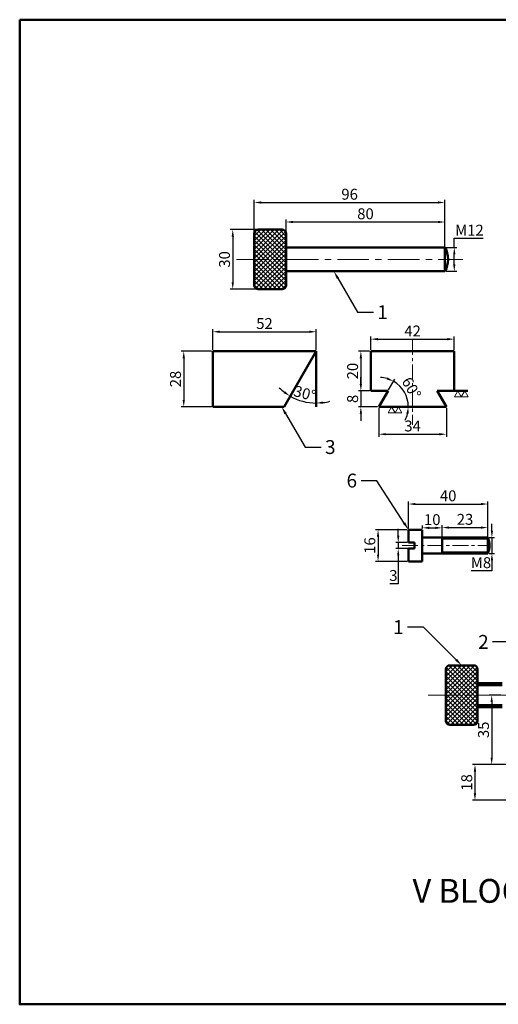
# Model space of a CAD drawing. Units: millimetres. Extents: x 10 to 613, y -226 to 271.
# Tile 1 of 4: x 10 to 251, y -226 to 271. Entities that reach past the tile are written whole.
import ezdxf
from ezdxf import colors
from ezdxf.entities.mleader import LeaderData, LeaderLine
from ezdxf.math import Vec2, Vec3

# ---------------------------------------------------------------- set-up
doc = ezdxf.new("R2010")
doc.units = ezdxf.units.MM
doc.header["$LTSCALE"] = 0.5
doc.linetypes.add('CENTER', pattern=[50.8, 31.75, -6.35, 6.35, -6.35])
for name, color, linetype, lineweight in [('M-CNTR', 1, 'CENTER', 18), ('M-DIMS', 2, 'Continuous', 25), ('M-HATC', 8, 'Continuous', 18), ('M-OUTL', 7, 'Continuous', 50), ('M-SYMB', 2, 'Continuous', 18), ('M-TEXT', 3, 'Continuous', 25), ('M-TTLB', 7, 'Continuous', 50)]:
    doc.layers.add(name, color=color, linetype=linetype, lineweight=lineweight)
doc.styles.get("Standard").update_dxf_attribs({"font": 'arial.ttf'})
doc.dimstyles.new('ISO-25', dxfattribs={"dimtxt": 5.5, "dimasz": 3.5, "dimexe": 1.25, "dimexo": 0.625, "dimtad": 1, "dimtoh": 1, "dimtxsty": 'Standard', "dimcen": 2.5, "dimadec": 0, "dimazin": 0, "dimtfac": 1, "dimtmove": 0, "dimatfit": 3, "dimfxl": 1, "dimarcsym": 0})

# ---------------------------------------------------------------- blocks, each defined once
blk = doc.blocks.new('*D1')
at = {"layer": 'Defpoints', "color": 0, "ltscale": 0.5, "transparency": 16777216}
for p in [(135.85, 164.86), (116.99, 134.86), (135.85, 134.86)]:
    blk.add_point(p, dxfattribs=at)
at = {"layer": 'M-DIMS', "color": 0, "lineweight": -2, "ltscale": 0.5, "transparency": 16777216}
for p, q in [((135.23, 164.86), (115.74, 164.86)), ((116.99, 161.36), (116.99, 138.36)), ((135.23, 134.86), (115.74, 134.86))]:
    blk.add_line(p, q, dxfattribs=at)
at = {"layer": 'M-DIMS', "color": 0, "ltscale": 0.5, "transparency": 16777216}
for points in [[(116.41, 161.36), (117.57, 161.36), (116.99, 164.86)], [(116.41, 138.36), (117.57, 138.36), (116.99, 134.86)]]:
    blk.add_solid(points, dxfattribs=at)
at = {"layer": 'M-DIMS', "color": 0, "ltscale": 0.5, "transparency": 16777216, "insert": (113.56, 149.86), "char_height": 5.5, "attachment_point": 5, "rotation": 90}
blk.add_mtext('30', dxfattribs=at)
blk = doc.blocks.new('*D2')
at = {"layer": 'Defpoints', "color": 0, "ltscale": 0.5, "transparency": 16777216}
for p in [(223.85, 168.71), (143.85, 155.86), (223.85, 155.86)]:
    blk.add_point(p, dxfattribs=at)
at = {"layer": 'M-DIMS', "color": 0, "lineweight": -2, "ltscale": 0.5, "transparency": 16777216}
for p, q in [((143.85, 156.49), (143.85, 169.96)), ((147.35, 168.71), (220.35, 168.71)), ((223.85, 156.49), (223.85, 169.96))]:
    blk.add_line(p, q, dxfattribs=at)
at = {"layer": 'M-DIMS', "color": 0, "ltscale": 0.5, "transparency": 16777216}
for points in [[(147.35, 169.29), (147.35, 168.12), (143.85, 168.71)], [(220.35, 169.29), (220.35, 168.12), (223.85, 168.71)]]:
    blk.add_solid(points, dxfattribs=at)
at = {"layer": 'M-DIMS', "color": 0, "ltscale": 0.5, "transparency": 16777216, "insert": (183.85, 172.14), "char_height": 5.5, "attachment_point": 5}
blk.add_mtext('80', dxfattribs=at)
blk = doc.blocks.new('*D3')
at = {"layer": 'Defpoints', "color": 0, "ltscale": 0.5, "transparency": 16777216}
for p in [(223.85, 178.55), (127.85, 149.86), (223.85, 149.86)]:
    blk.add_point(p, dxfattribs=at)
at = {"layer": 'M-DIMS', "color": 0, "lineweight": -2, "ltscale": 0.5, "transparency": 16777216}
for p, q in [((127.85, 150.49), (127.85, 179.8)), ((223.85, 150.49), (223.85, 179.8)), ((131.35, 178.55), (220.35, 178.55))]:
    blk.add_line(p, q, dxfattribs=at)
at = {"layer": 'M-DIMS', "color": 0, "ltscale": 0.5, "transparency": 16777216}
for points in [[(131.35, 179.13), (131.35, 177.96), (127.85, 178.55)], [(220.35, 179.13), (220.35, 177.96), (223.85, 178.55)]]:
    blk.add_solid(points, dxfattribs=at)
at = {"layer": 'M-DIMS', "color": 0, "ltscale": 0.5, "transparency": 16777216, "insert": (175.85, 181.98), "char_height": 5.5, "attachment_point": 5}
blk.add_mtext('96', dxfattribs=at)
blk = doc.blocks.new('*D4')
at = {"layer": 'Defpoints', "color": 0, "ltscale": 0.5, "transparency": 16777216}
for p in [(223.85, 155.86), (223.85, 143.86), (228.56, 143.86)]:
    blk.add_point(p, dxfattribs=at)
at = {"layer": 'M-DIMS', "color": 0, "lineweight": -2, "ltscale": 0.5, "transparency": 16777216}
for p, q in [((228.56, 155.86), (228.56, 160.48)), ((228.56, 160.48), (243.16, 160.48)), ((224.48, 155.86), (229.81, 155.86)), ((228.56, 147.36), (228.56, 152.36)), ((224.48, 143.86), (229.81, 143.86))]:
    blk.add_line(p, q, dxfattribs=at)
at = {"layer": 'M-DIMS', "color": 0, "ltscale": 0.5, "transparency": 16777216}
for points in [[(227.98, 152.36), (229.15, 152.36), (228.56, 155.86)], [(227.98, 147.36), (229.15, 147.36), (228.56, 143.86)]]:
    blk.add_solid(points, dxfattribs=at)
at = {"layer": 'M-DIMS', "color": 0, "ltscale": 0.5, "transparency": 16777216, "insert": (236.18, 163.87), "char_height": 5.5, "attachment_point": 5}
blk.add_mtext('M12', dxfattribs=at)
blk = doc.blocks.new('*D16')
at = {"layer": 'Defpoints', "color": 0, "ltscale": 0.5, "transparency": 16777216}
for p in [(106.98, 103.58), (92.32, 75.58), (106.98, 75.58)]:
    blk.add_point(p, dxfattribs=at)
at = {"layer": 'M-DIMS', "color": 0, "lineweight": -2, "ltscale": 0.5, "transparency": 16777216}
for p, q in [((106.36, 103.58), (91.07, 103.58)), ((92.32, 100.08), (92.32, 79.08)), ((106.36, 75.58), (91.07, 75.58))]:
    blk.add_line(p, q, dxfattribs=at)
at = {"layer": 'M-DIMS', "color": 0, "ltscale": 0.5, "transparency": 16777216}
for points in [[(91.73, 100.08), (92.9, 100.08), (92.32, 103.58)], [(91.73, 79.08), (92.9, 79.08), (92.32, 75.58)]]:
    blk.add_solid(points, dxfattribs=at)
at = {"layer": 'M-DIMS', "color": 0, "ltscale": 0.5, "transparency": 16777216, "insert": (88.88, 89.58), "char_height": 5.5, "attachment_point": 5, "rotation": 90}
blk.add_mtext('28', dxfattribs=at)
blk = doc.blocks.new('*D17')
at = {"layer": 'Defpoints', "color": 0, "ltscale": 0.5, "transparency": 16777216}
for p in [(158.98, 113.41), (106.98, 103.58), (158.98, 103.58)]:
    blk.add_point(p, dxfattribs=at)
at = {"layer": 'M-DIMS', "color": 0, "lineweight": -2, "ltscale": 0.5, "transparency": 16777216}
for p, q in [((106.98, 104.21), (106.98, 114.66)), ((158.98, 104.21), (158.98, 114.66)), ((110.48, 113.41), (155.48, 113.41))]:
    blk.add_line(p, q, dxfattribs=at)
at = {"layer": 'M-DIMS', "color": 0, "ltscale": 0.5, "transparency": 16777216}
for points in [[(110.48, 113.99), (110.48, 112.82), (106.98, 113.41)], [(155.48, 113.99), (155.48, 112.82), (158.98, 113.41)]]:
    blk.add_solid(points, dxfattribs=at)
at = {"layer": 'M-DIMS', "color": 0, "ltscale": 0.5, "transparency": 16777216, "insert": (132.98, 116.84), "char_height": 5.5, "attachment_point": 5}
blk.add_mtext('52', dxfattribs=at)
blk = doc.blocks.new('*D18')
at = {"layer": 'Defpoints', "color": 0, "ltscale": 0.5, "transparency": 16777216}
for p in [(158.98, 103.58), (158.98, 103.58), (142.82, 75.58), (150.05, 79.03), (158.98, 75.58)]:
    blk.add_point(p, dxfattribs=at)
at = {"layer": 'M-DIMS', "color": 0, "lineweight": -2, "ltscale": 0.5, "transparency": 16777216}
for start, end in [(224.6404, 232.3202), (240, 270), (277.6798, 285.3596)]:
    blk.add_arc((158.98, 103.58), 26.13, start, end, dxfattribs=at)
at = {"layer": 'M-DIMS', "color": 0, "ltscale": 0.5, "transparency": 16777216}
for points in [[(143.34, 83.39), (142.69, 82.42), (145.92, 80.95)], [(162.52, 77.1), (162.44, 78.27), (158.98, 77.45)]]:
    blk.add_solid(points, dxfattribs=at)
at = {"layer": 'M-DIMS', "color": 0, "ltscale": 0.5, "transparency": 16777216, "insert": (153.11, 81.66), "char_height": 5.5, "attachment_point": 5, "rotation": 345}
blk.add_mtext('30°', dxfattribs=at)
blk = doc.blocks.new('*D19')
at = {"layer": 'Defpoints', "color": 0, "ltscale": 0.5, "transparency": 16777216}
for p in [(195.19, 83.58), (204.52, 80.66), (190.57, 75.58), (190.57, 75.58), (224.57, 75.58)]:
    blk.add_point(p, dxfattribs=at)
at = {"layer": 'M-DIMS', "color": 0, "lineweight": -2, "ltscale": 0.5, "transparency": 16777216}
blk.add_line((195.5, 84.12), (198.61, 89.52), dxfattribs=at)
for start, end in [(73.541, 87.082), (0, 60), (332.918, 346.459)]:
    blk.add_arc((190.57, 75.58), 14.84, start, end, dxfattribs=at)
at = {"layer": 'M-DIMS', "color": 0, "ltscale": 0.5, "transparency": 16777216}
for points in [[(195, 90.35), (194.54, 89.28), (197.99, 88.44)], [(204.42, 72.18), (205.58, 72.04), (205.41, 75.58)]]:
    blk.add_solid(points, dxfattribs=at)
at = {"layer": 'M-DIMS', "color": 0, "ltscale": 0.5, "transparency": 16777216, "insert": (206.4, 84.72), "char_height": 5.5, "attachment_point": 5, "rotation": 300}
blk.add_mtext('60°', dxfattribs=at)
blk = doc.blocks.new('*D20')
at = {"layer": 'Defpoints', "color": 0, "ltscale": 0.5, "transparency": 16777216}
for p in [(186.57, 103.58), (181.51, 83.58), (186.57, 83.58)]:
    blk.add_point(p, dxfattribs=at)
at = {"layer": 'M-DIMS', "color": 0, "lineweight": -2, "ltscale": 0.5, "transparency": 16777216}
for p, q in [((185.94, 103.58), (180.26, 103.58)), ((181.51, 100.08), (181.51, 87.08)), ((185.94, 83.58), (180.26, 83.58))]:
    blk.add_line(p, q, dxfattribs=at)
at = {"layer": 'M-DIMS', "color": 0, "ltscale": 0.5, "transparency": 16777216}
for points in [[(180.92, 100.08), (182.09, 100.08), (181.51, 103.58)], [(180.92, 87.08), (182.09, 87.08), (181.51, 83.58)]]:
    blk.add_solid(points, dxfattribs=at)
at = {"layer": 'M-DIMS', "color": 0, "ltscale": 0.5, "transparency": 16777216, "insert": (178.07, 93.58), "char_height": 5.5, "attachment_point": 5, "rotation": 90}
blk.add_mtext('20', dxfattribs=at)
blk = doc.blocks.new('*D21')
at = {"layer": 'Defpoints', "color": 0, "ltscale": 0.5, "transparency": 16777216}
for p in [(186.57, 83.58), (181.51, 75.58), (190.57, 75.58)]:
    blk.add_point(p, dxfattribs=at)
at = {"layer": 'M-DIMS', "color": 0, "lineweight": -2, "ltscale": 0.5, "transparency": 16777216}
for p, q in [((181.51, 87.08), (181.51, 90.58)), ((185.94, 83.58), (180.26, 83.58)), ((181.51, 83.58), (181.51, 75.58)), ((189.94, 75.58), (180.26, 75.58)), ((181.51, 72.08), (181.51, 68.58))]:
    blk.add_line(p, q, dxfattribs=at)
at = {"layer": 'M-DIMS', "color": 0, "ltscale": 0.5, "transparency": 16777216}
for points in [[(180.92, 87.08), (182.09, 87.08), (181.51, 83.58)], [(180.92, 72.08), (182.09, 72.08), (181.51, 75.58)]]:
    blk.add_solid(points, dxfattribs=at)
at = {"layer": 'M-DIMS', "color": 0, "ltscale": 0.5, "transparency": 16777216, "insert": (178.07, 79.58), "char_height": 5.5, "attachment_point": 5, "rotation": 90}
blk.add_mtext('8', dxfattribs=at)
blk = doc.blocks.new('*D22')
at = {"layer": 'Defpoints', "color": 0, "ltscale": 0.5, "transparency": 16777216}
for p in [(228.57, 109.68), (186.57, 103.58), (228.57, 103.58)]:
    blk.add_point(p, dxfattribs=at)
at = {"layer": 'M-DIMS', "color": 0, "lineweight": -2, "ltscale": 0.5, "transparency": 16777216}
for p, q in [((186.57, 104.21), (186.57, 110.93)), ((190.07, 109.68), (225.07, 109.68)), ((228.57, 104.21), (228.57, 110.93))]:
    blk.add_line(p, q, dxfattribs=at)
at = {"layer": 'M-DIMS', "color": 0, "ltscale": 0.5, "transparency": 16777216}
for points in [[(190.07, 110.26), (190.07, 109.09), (186.57, 109.68)], [(225.07, 110.26), (225.07, 109.09), (228.57, 109.68)]]:
    blk.add_solid(points, dxfattribs=at)
at = {"layer": 'M-DIMS', "color": 0, "ltscale": 0.5, "transparency": 16777216, "insert": (207.57, 113.06), "char_height": 5.5, "attachment_point": 5}
blk.add_mtext('42', dxfattribs=at)
blk = doc.blocks.new('*D23')
at = {"layer": 'Defpoints', "color": 0, "ltscale": 0.5, "transparency": 16777216}
for p in [(190.57, 75.58), (224.57, 75.58), (224.57, 61.76)]:
    blk.add_point(p, dxfattribs=at)
at = {"layer": 'M-DIMS', "color": 0, "lineweight": -2, "ltscale": 0.5, "transparency": 16777216}
for p, q in [((190.57, 74.96), (190.57, 60.51)), ((224.57, 74.96), (224.57, 60.51)), ((194.07, 61.76), (221.07, 61.76))]:
    blk.add_line(p, q, dxfattribs=at)
at = {"layer": 'M-DIMS', "color": 0, "ltscale": 0.5, "transparency": 16777216}
for points in [[(194.07, 62.34), (194.07, 61.18), (190.57, 61.76)], [(221.07, 62.34), (221.07, 61.18), (224.57, 61.76)]]:
    blk.add_solid(points, dxfattribs=at)
at = {"layer": 'M-DIMS', "color": 0, "ltscale": 0.5, "transparency": 16777216, "insert": (207.57, 65.2), "char_height": 5.5, "attachment_point": 5}
blk.add_mtext('34', dxfattribs=at)
blk = doc.blocks.new('*D46')
at = {"layer": 'Defpoints', "color": 0, "ltscale": 0.5, "transparency": 16777216}
for p in [(245.47, 26.59), (205.47, 13.65), (245.47, 9.15)]:
    blk.add_point(p, dxfattribs=at)
at = {"layer": 'M-DIMS', "color": 0, "lineweight": -2, "ltscale": 0.5, "transparency": 16777216}
for p, q in [((205.47, 14.27), (205.47, 27.84)), ((208.97, 26.59), (241.97, 26.59)), ((245.47, 9.77), (245.47, 27.84))]:
    blk.add_line(p, q, dxfattribs=at)
at = {"layer": 'M-DIMS', "color": 0, "ltscale": 0.5, "transparency": 16777216}
for points in [[(208.97, 27.17), (208.97, 26), (205.47, 26.59)], [(241.97, 27.17), (241.97, 26), (245.47, 26.59)]]:
    blk.add_solid(points, dxfattribs=at)
at = {"layer": 'M-DIMS', "color": 0, "ltscale": 0.5, "transparency": 16777216, "insert": (225.47, 30.02), "char_height": 5.5, "attachment_point": 5}
blk.add_mtext('40', dxfattribs=at)
blk = doc.blocks.new('*D47')
at = {"layer": 'Defpoints', "color": 0, "ltscale": 0.5, "transparency": 16777216}
for p in [(245.47, 14.71), (222.47, 9.65), (245.47, 9.65)]:
    blk.add_point(p, dxfattribs=at)
at = {"layer": 'M-DIMS', "color": 0, "lineweight": -2, "ltscale": 0.5, "transparency": 16777216}
for p, q in [((222.47, 10.27), (222.47, 15.96)), ((245.47, 10.27), (245.47, 15.96)), ((225.97, 14.71), (241.97, 14.71))]:
    blk.add_line(p, q, dxfattribs=at)
at = {"layer": 'M-DIMS', "color": 0, "ltscale": 0.5, "transparency": 16777216}
for points in [[(225.97, 15.3), (225.97, 14.13), (222.47, 14.71)], [(241.97, 15.3), (241.97, 14.13), (245.47, 14.71)]]:
    blk.add_solid(points, dxfattribs=at)
at = {"layer": 'M-DIMS', "color": 0, "ltscale": 0.5, "transparency": 16777216, "insert": (233.97, 18.15), "char_height": 5.5, "attachment_point": 5}
blk.add_mtext('23', dxfattribs=at)
blk = doc.blocks.new('*D48')
at = {"layer": 'Defpoints', "color": 0, "ltscale": 0.5, "transparency": 16777216}
for p in [(212.47, 13.65), (222.47, 14.58), (222.47, 9.65)]:
    blk.add_point(p, dxfattribs=at)
at = {"layer": 'M-DIMS', "color": 0, "lineweight": -2, "ltscale": 0.5, "transparency": 16777216}
for p, q in [((212.47, 14.27), (212.47, 15.83)), ((222.47, 10.27), (222.47, 15.83)), ((215.97, 14.58), (218.97, 14.58))]:
    blk.add_line(p, q, dxfattribs=at)
at = {"layer": 'M-DIMS', "color": 0, "ltscale": 0.5, "transparency": 16777216}
for points in [[(215.97, 15.16), (215.97, 13.99), (212.47, 14.58)], [(218.97, 15.16), (218.97, 13.99), (222.47, 14.58)]]:
    blk.add_solid(points, dxfattribs=at)
at = {"layer": 'M-DIMS', "color": 0, "ltscale": 0.5, "transparency": 16777216, "insert": (217.47, 18.01), "char_height": 5.5, "attachment_point": 5}
blk.add_mtext('10', dxfattribs=at)
blk = doc.blocks.new('*D49')
at = {"layer": 'Defpoints', "color": 0, "ltscale": 0.5, "transparency": 16777216}
for p in [(205.47, 13.65), (190.17, -2.35), (205.47, -2.35)]:
    blk.add_point(p, dxfattribs=at)
at = {"layer": 'M-DIMS', "color": 0, "lineweight": -2, "ltscale": 0.5, "transparency": 16777216}
for p, q in [((204.84, 13.65), (188.92, 13.65)), ((190.17, 10.15), (190.17, 1.15)), ((204.84, -2.35), (188.92, -2.35))]:
    blk.add_line(p, q, dxfattribs=at)
at = {"layer": 'M-DIMS', "color": 0, "ltscale": 0.5, "transparency": 16777216}
for points in [[(189.59, 10.15), (190.75, 10.15), (190.17, 13.65)], [(189.59, 1.15), (190.75, 1.15), (190.17, -2.35)]]:
    blk.add_solid(points, dxfattribs=at)
at = {"layer": 'M-DIMS', "color": 0, "ltscale": 0.5, "transparency": 16777216, "insert": (186.74, 5.65), "char_height": 5.5, "attachment_point": 5, "rotation": 90}
blk.add_mtext('16', dxfattribs=at)
blk = doc.blocks.new('*D50')
at = {"layer": 'Defpoints', "color": 0, "ltscale": 0.5, "transparency": 16777216}
for p in [(205.47, 7.15), (200.33, 4.15), (206.97, 4.15)]:
    blk.add_point(p, dxfattribs=at)
at = {"layer": 'M-DIMS', "color": 0, "lineweight": -2, "ltscale": 0.5, "transparency": 16777216}
for p, q in [((200.33, 10.65), (200.33, 14.15)), ((204.84, 7.15), (199.08, 7.15)), ((200.33, 7.15), (200.33, 4.15)), ((206.34, 4.15), (199.08, 4.15)), ((200.33, 0.65), (200.33, -13.57)), ((200.33, -13.57), (196.1, -13.57))]:
    blk.add_line(p, q, dxfattribs=at)
at = {"layer": 'M-DIMS', "color": 0, "ltscale": 0.5, "transparency": 16777216}
for points in [[(199.74, 10.65), (200.91, 10.65), (200.33, 7.15)], [(199.74, 0.65), (200.91, 0.65), (200.33, 4.15)]]:
    blk.add_solid(points, dxfattribs=at)
at = {"layer": 'M-DIMS', "color": 0, "ltscale": 0.5, "transparency": 16777216, "insert": (197.9, -10.13), "char_height": 5.5, "attachment_point": 5}
blk.add_mtext('3', dxfattribs=at)
blk = doc.blocks.new('*D51')
at = {"layer": 'Defpoints', "color": 0, "ltscale": 0.5, "transparency": 16777216}
for p in [(245.47, 9.65), (245.47, 1.65), (247.51, 1.65)]:
    blk.add_point(p, dxfattribs=at)
at = {"layer": 'M-DIMS', "color": 0, "lineweight": -2, "ltscale": 0.5, "transparency": 16777216}
for p, q in [((247.51, 13.15), (247.51, 16.65)), ((246.09, 9.65), (248.76, 9.65)), ((247.51, 9.65), (247.51, 1.65)), ((246.09, 1.65), (248.76, 1.65)), ((247.51, -1.85), (247.51, -7.12)), ((247.51, -7.12), (237.12, -7.12))]:
    blk.add_line(p, q, dxfattribs=at)
at = {"layer": 'M-DIMS', "color": 0, "ltscale": 0.5, "transparency": 16777216}
for points in [[(246.93, 13.15), (248.1, 13.15), (247.51, 9.65)], [(246.93, -1.85), (248.1, -1.85), (247.51, 1.65)]]:
    blk.add_solid(points, dxfattribs=at)
at = {"layer": 'M-DIMS', "color": 0, "ltscale": 0.5, "transparency": 16777216, "insert": (242.01, -3.68), "char_height": 5.5, "attachment_point": 5}
blk.add_mtext('M8', dxfattribs=at)
blk = doc.blocks.new('*D52')
at = {"layer": 'Defpoints', "color": 0, "ltscale": 0.5, "transparency": 16777216}
for p in [(274.69, -104.71), (238.97, -122.71), (274.69, -122.71)]:
    blk.add_point(p, dxfattribs=at)
at = {"layer": 'M-DIMS', "color": 0, "lineweight": -2, "ltscale": 0.5, "transparency": 16777216}
for p, q in [((274.07, -104.71), (237.72, -104.71)), ((238.97, -108.21), (238.97, -119.21)), ((274.07, -122.71), (237.72, -122.71))]:
    blk.add_line(p, q, dxfattribs=at)
at = {"layer": 'M-DIMS', "color": 0, "ltscale": 0.5, "transparency": 16777216}
for points in [[(238.39, -108.21), (239.56, -108.21), (238.97, -104.71)], [(238.39, -119.21), (239.56, -119.21), (238.97, -122.71)]]:
    blk.add_solid(points, dxfattribs=at)
at = {"layer": 'M-DIMS', "color": 0, "ltscale": 0.5, "transparency": 16777216, "insert": (235.54, -113.71), "char_height": 5.5, "attachment_point": 5, "rotation": 90}
blk.add_mtext('18', dxfattribs=at)
blk = doc.blocks.new('*D53')
at = {"layer": 'Defpoints', "color": 0, "ltscale": 0.5, "transparency": 16777216}
for p in [(252.69, -69.71), (247.41, -104.71), (252.69, -104.71)]:
    blk.add_point(p, dxfattribs=at)
at = {"layer": 'M-DIMS', "color": 0, "lineweight": -2, "ltscale": 0.5, "transparency": 16777216}
for p, q in [((252.07, -69.71), (246.16, -69.71)), ((247.41, -73.21), (247.41, -101.21)), ((252.07, -104.71), (246.16, -104.71))]:
    blk.add_line(p, q, dxfattribs=at)
at = {"layer": 'M-DIMS', "color": 0, "ltscale": 0.5, "transparency": 16777216}
for points in [[(246.83, -73.21), (247.99, -73.21), (247.41, -69.71)], [(246.83, -101.21), (247.99, -101.21), (247.41, -104.71)]]:
    blk.add_solid(points, dxfattribs=at)
at = {"layer": 'M-DIMS', "color": 0, "ltscale": 0.5, "transparency": 16777216, "insert": (243.98, -87.21), "char_height": 5.5, "attachment_point": 5, "rotation": 90}
blk.add_mtext('35', dxfattribs=at)
blk = doc.blocks.new('SYM-SURF-FINISH')
at = {"ltscale": 0.5}
for points in [[(230.36, 83.58), (228.63, 80.58), (232.09, 80.58)], [(233.82, 83.58), (232.09, 80.58), (235.55, 80.58)]]:
    blk.add_lwpolyline(points, close=True, dxfattribs=at)

msp = doc.modelspace()

# ---------------------------------------------------------------- hatches: boundary and pattern name
at = {"layer": 'M-HATC', "ltscale": 0.5}
h = msp.add_hatch(dxfattribs=at)
h.set_pattern_fill('ANSI37', color=256, scale=0.5)
h.paths.add_polyline_path([(143.854, 149.862), (127.854, 149.862), (127.854, 136.862, 0.4142136), (129.854, 134.862), (141.854, 134.862, 0.4142136), (143.854, 136.862)])
h.paths.add_polyline_path([(143.854, 162.862, 0.4142136), (141.854, 164.862), (129.854, 164.862, 0.4142136), (127.854, 162.862), (127.854, 149.862), (143.854, 149.862)])
h = msp.add_hatch(dxfattribs=at)
h.set_pattern_fill('ANSI37', color=256, scale=0.5)
h.set_pattern_definition([(45, (96.4558, -219.5703), (-1.122532, 1.122532), []), (135, (96.4558, -219.5703), (-1.122532, -1.122532), [])])
h.paths.add_polyline_path([(240.31, -69.708), (224.31, -69.708), (224.31, -82.708, 0.4142136), (226.31, -84.708), (238.31, -84.708, 0.4142136), (240.31, -82.708)])
h.paths.add_polyline_path([(240.31, -56.708, 0.4142136), (238.31, -54.708), (226.31, -54.708, 0.4142136), (224.31, -56.708), (224.31, -69.708), (240.31, -69.708)])

# ---------------------------------------------------------------- linework, layer by layer
at = {"layer": 'M-CNTR'}
for p, q in [((118.928, 149.862), (232.885, 149.862)), ((215.384, -69.708), (329.34, -69.708))]:
    msp.add_line(p, q, dxfattribs=at)
at = {"layer": 'M-CNTR', "ltscale": 0.5}
for p, q in [((207.567, 109.636), (207.567, 66.504)), ((202.3, 5.649), (245.465, 5.649))]:
    msp.add_line(p, q, dxfattribs=at)
at = {"layer": 'M-OUTL'}
for p, q in [((141.854, 164.862), (129.854, 164.862)), ((127.854, 162.862), (127.854, 136.862)), ((143.854, 136.862), (143.854, 162.862)), ((223.854, 155.862), (143.854, 155.862)), ((223.854, 149.862), (223.854, 155.862)), ((223.854, 149.862), (223.854, 143.862)), ((223.854, 143.862), (143.854, 143.862)), ((129.854, 134.862), (141.854, 134.862)), ((224.31, -56.708), (224.31, -82.708)), ((238.31, -54.708), (226.31, -54.708)), ((240.31, -82.708), (240.31, -56.708)), ((252.691, -63.708), (240.31, -63.708)), ((252.691, -64.708), (240.31, -64.708)), ((252.691, -74.708), (240.31, -74.708)), ((252.691, -75.708), (240.31, -75.708)), ((226.31, -84.708), (238.31, -84.708))]:
    msp.add_line(p, q, dxfattribs=at)
at = {"layer": 'M-OUTL', "ltscale": 0.5}
for p, q in [((106.985, 103.582), (106.985, 75.582)), ((106.985, 103.582), (158.985, 103.582)), ((158.985, 103.582), (142.819, 75.582)), ((158.985, 103.582), (158.985, 75.582)), ((186.567, 103.582), (186.567, 83.582)), ((228.567, 103.582), (186.567, 103.582)), ((228.567, 83.582), (228.567, 103.582)), ((186.567, 83.582), (195.186, 83.582)), ((190.567, 75.582), (195.186, 83.582)), ((224.567, 75.582), (219.949, 83.582)), ((219.949, 83.582), (228.567, 83.582)), ((228.567, 83.582), (235.461, 83.582)), ((142.819, 75.582), (106.985, 75.582)), ((190.567, 75.582), (224.567, 75.582)), ((205.465, 13.649), (205.465, 7.149)), ((212.465, 13.649), (205.465, 13.649)), ((212.465, -2.351), (212.465, 13.649)), ((205.465, 7.149), (208.465, 7.149)), ((208.465, 7.149), (208.465, 4.149)), ((245.465, 9.649), (212.465, 9.649)), ((222.465, 1.649), (222.465, 9.649)), ((245.465, 9.149), (222.465, 9.149)), ((245.465, 1.649), (245.465, 9.649)), ((208.465, 4.149), (205.465, 4.149)), ((205.465, 4.149), (205.465, -2.351)), ((245.465, 1.649), (212.465, 1.649)), ((245.465, 2.149), (222.465, 2.149)), ((205.465, -2.351), (212.465, -2.351))]:
    msp.add_line(p, q, dxfattribs=at)
at = {"layer": 'M-OUTL'}
for centre, start, end in [((129.854, 162.862), 90, 180), ((141.854, 162.862), 0, 90), ((129.854, 136.862), 180, 270), ((141.854, 136.862), 270, 0), ((226.31, -56.708), 90, 180), ((238.31, -56.708), 0, 90), ((226.31, -82.708), 180, 270), ((238.31, -82.708), 270, 0)]:
    msp.add_arc(centre, 2, start, end, dxfattribs=at)
at = {"layer": 'M-OUTL', "ltscale": 0.5}
for centre, radius, start, end in [((213.462, 149.862), 12, 330, 30), ((237.106, 5.649), 9.267, 334.42974, 25.57026)]:
    msp.add_arc(centre, radius, start, end, dxfattribs=at)
at = {"layer": 'M-TTLB', "ltscale": 0.5}
msp.add_lwpolyline([(9.692, 270.659), (613.416, 270.659), (613.416, -225.522), (9.692, -225.522)], close=True, dxfattribs=at)

# ---------------------------------------------------------------- block references
at = {"layer": 'M-SYMB'}
for p in [(0, 0), (-33.357, -8)]:
    msp.add_blockref('SYM-SURF-FINISH', p, dxfattribs=at)

# ---------------------------------------------------------------- texts
at = {"layer": 'M-TEXT', "ltscale": 0.5, "insert": (207.538, -162.361), "char_height": 12, "attachment_point": 1}
msp.add_mtext_dynamic_manual_height_columns('V BLOCK ADJUSTABLE SUPPORT', width=297.62232, gutter_width=12.5, heights=[0], dxfattribs=at)

# ---------------------------------------------------------------- dimensions: what is measured, and where the dimension line sits
at = {"layer": 'M-DIMS', "ltscale": 0.5}
for base, p1, p2, picture, middle in [((223.854, 178.547), (127.854, 149.862), (223.854, 149.862), '*D3', (175.854, 181.98)), ((223.854, 168.708), (143.854, 155.862), (223.854, 155.862), '*D2', (183.854, 172.141)), ((158.985, 113.405), (106.985, 103.582), (158.985, 103.582), '*D17', (132.985, 116.838)), ((228.567, 109.678), (186.567, 103.582), (228.567, 103.582), '*D22', (207.567, 113.064)), ((224.567, 61.76), (190.567, 75.582), (224.567, 75.582), '*D23', (207.567, 65.195)), ((245.465, 26.586), (205.465, 13.649), (245.465, 9.149), '*D46', (225.465, 30.019)), ((222.465, 14.576), (212.465, 13.649), (222.465, 9.649), '*D48', (217.465, 18.009)), ((245.465, 14.713), (222.465, 9.649), (245.465, 9.649), '*D47', (233.965, 18.148))]:
    dim = msp.add_linear_dim(base=base, p1=p1, p2=p2, dimstyle='ISO-25', override={"dimclrd": 0, "dimclre": 0, "dimclrt": 0}, dxfattribs=at)
    dim.commit()
    dim.dimension.update_dxf_attribs({"geometry": picture, "text_midpoint": middle})
for base, p1, p2, picture, middle in [((116.991, 134.862), (135.854, 164.862), (135.854, 134.862), '*D1', (113.556, 149.862)), ((92.316, 75.582), (106.985, 103.582), (106.985, 75.582), '*D16', (88.882, 89.582)), ((181.508, 83.582), (186.567, 103.582), (186.567, 83.582), '*D20', (178.075, 93.582)), ((181.508, 75.582), (186.567, 83.582), (190.567, 75.582), '*D21', (178.075, 79.582)), ((190.17, -2.351), (205.465, 13.649), (205.465, -2.351), '*D49', (186.737, 5.649)), ((247.411, -104.708), (252.691, -69.708), (252.691, -104.708), '*D53', (243.976, -87.208)), ((238.972, -122.708), (274.691, -104.708), (274.691, -122.708), '*D52', (235.539, -113.708))]:
    dim = msp.add_linear_dim(base=base, p1=p1, p2=p2, angle=90, dimstyle='ISO-25', override={"dimclrd": 0, "dimclre": 0, "dimclrt": 0}, dxfattribs=at)
    dim.commit()
    dim.dimension.update_dxf_attribs({"geometry": picture, "text_midpoint": middle})
for base, p1, p2, picture, middle in [((228.565, 143.862), (223.854, 155.862), (223.854, 143.862), '*D4', (236.175, 160.48)), ((247.513, 1.649), (245.465, 9.649), (245.465, 1.649), '*D51', (242.005, -7.116))]:
    dim = msp.add_linear_dim(base=base, p1=p1, p2=p2, angle=90, text='M<>', dimstyle='ISO-25', override={"dimclrd": 0, "dimclre": 0, "dimclrt": 0}, dxfattribs=at)
    dim.commit()
    dim.dimension.update_dxf_attribs({"geometry": picture, "text_midpoint": middle, "dimtype": 160})
for base, line1, line2, picture, middle in [((150.047, 79.027), ((158.985, 103.582), (158.985, 75.582)), ((158.985, 103.582), (142.819, 75.582)), '*D18', (153.11, 81.659)), ((204.516, 80.659), ((190.567, 75.582), (224.567, 75.582)), ((190.567, 75.582), (195.186, 83.582)), '*D19', (206.396, 84.721))]:
    dim = msp.add_angular_dim_2l(base=base, line1=line1, line2=line2, dimstyle='ISO-25', override={"dimclrd": 0, "dimclre": 0, "dimclrt": 0}, dxfattribs=at)
    dim.commit()
    dim.dimension.update_dxf_attribs({"geometry": picture, "text_midpoint": middle})
dim = msp.add_linear_dim(base=(200.326, 4.149), p1=(205.465, 7.149), p2=(206.965, 4.149), angle=90, dimstyle='ISO-25', override={"dimclrd": 0, "dimclre": 0, "dimclrt": 0}, dxfattribs=at)
dim.commit()
dim.dimension.update_dxf_attribs({"geometry": '*D50', "text_midpoint": (197.9, -13.567), "dimtype": 160})

# ---------------------------------------------------------------- leaders
ml = msp.add_multileader_mtext('Standard', dxfattribs=at)
ml.set_content('1', color=256)
ml.set_leader_properties()
ml.build(insert=Vec2(0, 0))
ctx = ml.context
ctx.base_point, ctx.char_height, ctx.plane_origin = Vec3(187.804, 123.274), 7, Vec3(167.918, 143.862)
notes = []
notes.append((ctx, [(0, (1, 1, 0), (179.804, 123.274), (1, 0), 8, [(0, [(167.918, 143.862)], 0, [])])]))
ctx.mtext.insert, ctx.mtext.flow_direction = Vec3(189.804, 126.774), 5
ml = msp.add_multileader_mtext('Standard', dxfattribs=at)
ml.set_content('3', color=256)
ml.set_leader_properties()
ml.build(insert=Vec2(0, 0))
ctx = ml.context
ctx.base_point, ctx.char_height, ctx.plane_origin = Vec3(161.478, 55.232), 7, Vec3(141.591, 75.821)
notes.append((ctx, [(0, (1, 1, 0), (153.478, 55.232), (1, 0), 8, [(0, [(141.591, 75.582)], 0, [])])]))
ctx.mtext.insert, ctx.mtext.flow_direction = Vec3(163.478, 58.794), 5
ml = msp.add_multileader_mtext('Standard', dxfattribs=at)
ml.set_content('6', color=256)
ml.set_leader_properties()
ml.build(insert=Vec2(0, 0))
ctx = ml.context
ctx.base_point, ctx.char_height, ctx.plane_origin = Vec3(172.978, 38.346), 7, Vec3(205.465, 13.649)
ctx.text_align_type = 2
notes.append((ctx, [(0, (1, 1, 0), (189.6, 38.346), (-1, 0), 8, [(0, [(205.465, 13.649)], 0, [])])]))
ctx.mtext.insert, ctx.mtext.alignment, ctx.mtext.flow_direction = Vec3(179.6, 41.906), 3, 5
ml = msp.add_multileader_mtext('Standard', dxfattribs=at)
ml.set_content('1', color=256)
ml.set_leader_properties()
ml.build(insert=Vec2(0, 0))
ctx = ml.context
ctx.base_point, ctx.char_height, ctx.plane_origin = Vec3(198.457, -35.433), 7, Vec3(232.31, -54.708)
ctx.text_align_type = 2
notes.append((ctx, [(0, (1, 1, 0), (213.035, -35.433), (-1, 0), 8, [(0, [(232.31, -54.708)], 0, [])])]))
ctx.mtext.insert, ctx.mtext.width, ctx.mtext.alignment, ctx.mtext.flow_direction = Vec3(203.035, -31.933), 2.57844, 3, 5
ml = msp.add_multileader_mtext('Standard', dxfattribs=at)
ml.set_content('2', color=256)
ml.set_leader_properties()
ml.build(insert=Vec2(0, 0))
ctx = ml.context
ctx.base_point, ctx.char_height, ctx.plane_origin = Vec3(239.253, -42.893), 7, Vec3(263.676, -59.708)
ctx.text_align_type = 2
notes.append((ctx, [(0, (1, 1, 0), (255.89, -42.893), (-1, 0), 8, [(0, [(263.676, -59.708)], 0, [])])]))
ctx.mtext.insert, ctx.mtext.alignment, ctx.mtext.flow_direction = Vec3(245.89, -39.393), 3, 5
for ctx, leaders in notes:
    for number, flags, end, landing, length, lines in leaders:
        leader = LeaderData()
        leader.index, (leader.has_last_leader_line, leader.has_dogleg_vector, leader.attachment_direction) = number, flags
        leader.last_leader_point, leader.dogleg_vector, leader.dogleg_length = Vec3(end), Vec3(landing), length
        for number, points, colour, breaks in lines:
            line = LeaderLine()
            line.index, line.vertices, line.color, line.breaks = number, Vec3.list(points), colors.encode_raw_color(colour), breaks
            leader.lines.append(line)
        ctx.leaders.append(leader)

doc.saveas('drawing.dxf')
